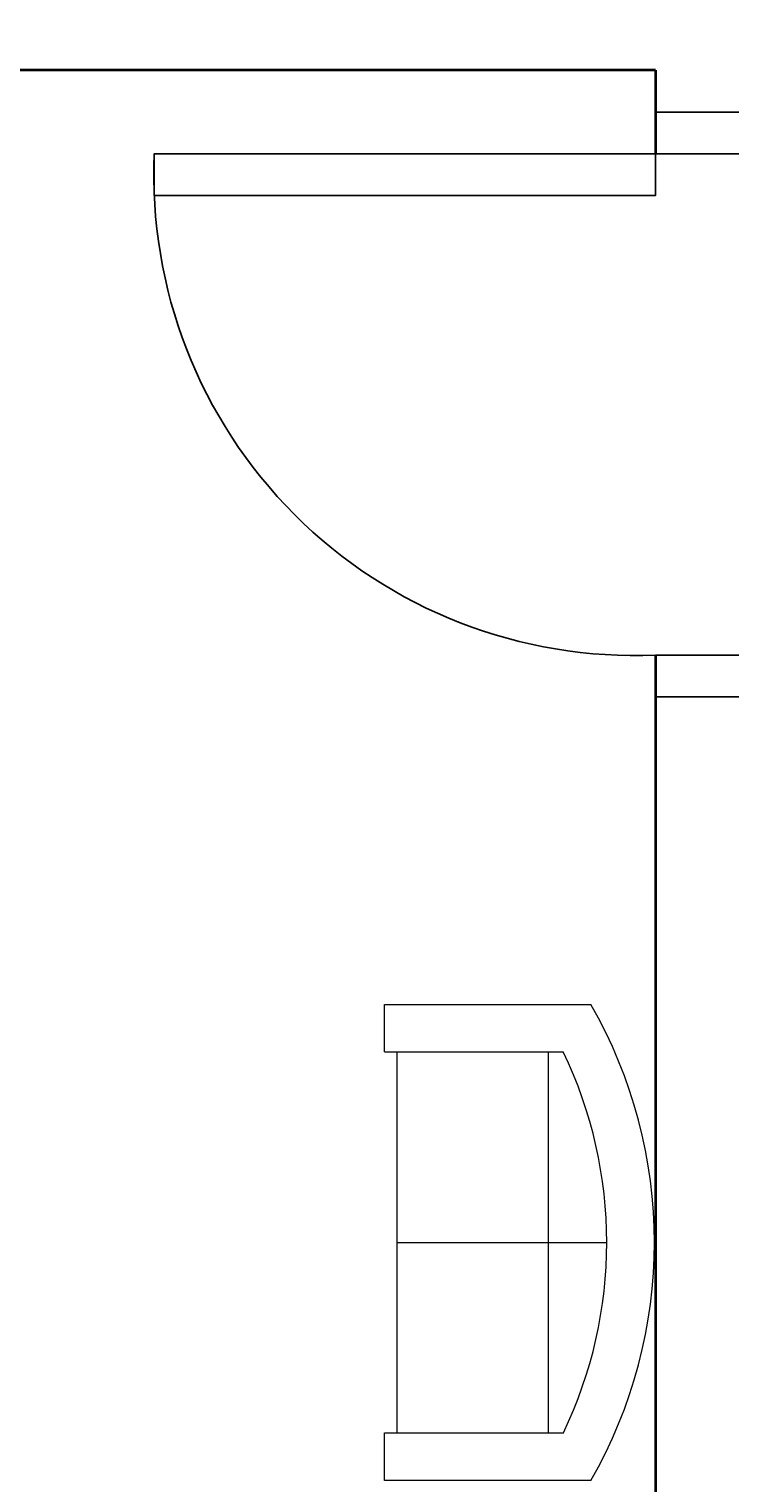
# Model space of a CAD drawing. Units: inches. Extents: x 4159 to 4826, y 299 to 1026.
# Tile 26 of 37: x 4402 to 4453, y 559 to 663. Entities that reach past the tile are written whole.
import ezdxf

# ---------------------------------------------------------------- set-up
doc = ezdxf.new("R2010")
doc.units = ezdxf.units.IN
for name, color, linetype, lineweight in [('A-ANNO-DIMS', 2, 'Continuous', 18), ('A-DOOR', 4, 'Continuous', 25), ('A-FURN', 8, 'Continuous', 18), ('A-WALL', 7, 'Continuous', 35)]:
    doc.layers.add(name, color=color, linetype=linetype, lineweight=lineweight)
doc.styles.get("Standard").update_dxf_attribs({"font": 'arial.ttf'})
doc.dimstyles.get("Standard").update_dxf_attribs({"dimtxt": 0.18, "dimasz": 0.18, "dimexe": 0.18, "dimexo": 0.0625, "dimgap": 0.09, "dimtad": 0, "dimtih": 1, "dimtoh": 1, "dimdec": 4, "dimzin": 0, "dimdsep": 46, "dimtxsty": 'Standard', "dimcen": 0.09, "dimadec": 0, "dimazin": 0, "dimtfac": 1, "dimtdec": 4, "dimtofl": 0, "dimtmove": 0, "dimatfit": 3, "dimfxl": 1, "dimtolj": 1, "dimtzin": 0, "dimarcsym": 0})

# ---------------------------------------------------------------- blocks, each defined once
blk = doc.blocks.new('Sofa - Roundback Loveseat 5 ft.')
for p, q in [((0, -32.44198), (0, -5.99998)), ((-24, -33.99998), (-24, -11.46958)), ((24.00004, -33.99998), (24.00004, -11.46958)), ((-23.9998, -13.38178), (23.99986, -13.38178)), ((-24, -32.44198), (24.00004, -32.44198))]:
    blk.add_line(p, q)
for points in [[(-24, -33.99998), (-30, -33.99998), (-30, -7.99998)], [(30.00004, -7.99998), (30.00004, -33.99998), (24.00004, -33.99998)]]:
    blk.add_lwpolyline(points)
for centre, radius, start, end in [((0, -60.24998), 60.24998, 60.13715, 119.8628), ((0, -61.38438), 55.38444, 64.32083, 115.6792)]:
    blk.add_arc(centre, radius, start, end)
blk = doc.blocks.new('DOOR-SWING-36IN')
blk.add_lwpolyline([(0, 0), (-3, 0), (-3, 36), (0, 36)], close=True)
blk.add_arc((-1.5, 1.5), 34.53, 87.5104, 182.4896)
blk = doc.blocks.new('DOOR-FRAME-36IN')
for p, q in [((0, 6), (0, 0)), ((3, 6), (3, 0)), ((39, 6), (39, 0)), ((42, 6), (42, 0))]:
    blk.add_line(p, q)
blk = doc.blocks.new('*D44')
at = {"layer": 'A-ANNO-DIMS', "color": 0, "lineweight": -2, "transparency": 16777216}
for p, q in [((4287.26, 963.09), (4158.88, 963.09)), ((4159.06, 962.91), (4159.06, 647.83)), ((4159.06, 332.38), (4159.06, 647.46)), ((4447.25, 332.2), (4158.88, 332.2))]:
    blk.add_line(p, q, dxfattribs=at)
at = {"layer": 'A-ANNO-DIMS', "color": 0, "transparency": 16777216}
for points in [[(4159.03, 962.91), (4159.09, 962.91), (4159.06, 963.09)], [(4159.03, 332.38), (4159.09, 332.38), (4159.06, 332.2)]]:
    blk.add_solid(points, dxfattribs=at)
at = {"layer": 'Defpoints', "color": 0, "transparency": 16777216}
for p in [(4287.33, 963.09), (4159.06, 332.2), (4447.31, 332.2)]:
    blk.add_point(p, dxfattribs=at)
at = {"layer": 'A-ANNO-DIMS', "color": 0, "transparency": 16777216, "insert": (4159.06, 647.64), "char_height": 0.18, "attachment_point": 5}
blk.add_mtext('\\A1;630.9', dxfattribs=at)

msp = doc.modelspace()

# ---------------------------------------------------------------- linework, layer by layer
at = {"layer": 'A-WALL'}
for p, q in [((4447.31, 660.254), (4201.31, 660.254)), ((4447.31, 660.254), (4447.31, 654.254)), ((4447.31, 618.254), (4447.31, 539.254))]:
    msp.add_line(p, q, dxfattribs=at)

# ---------------------------------------------------------------- block references
at = {"layer": 'A-DOOR'}
for name, p, rotation in [('DOOR-FRAME-36IN', (4453.31, 615.254), 90.0000000000003), ('DOOR-SWING-36IN', (4447.31, 654.254), 89.99999999999957)]:
    msp.add_blockref(name, p, dxfattribs=dict(at, rotation=rotation))
at = {"layer": 'A-FURN', "xscale": 0.5700533147329089, "yscale": 0.5700533147329089, "zscale": 0.5700533147329089, "rotation": 270}
msp.add_blockref('Sofa - Roundback Loveseat 5 ft.', (4447.235, 576.069), dxfattribs=at)

# ---------------------------------------------------------------- dimensions: what is measured, and where the dimension line sits
at = {"layer": 'A-ANNO-DIMS'}
dim = msp.add_linear_dim(base=(4159.06, 332.195), p1=(4287.326, 963.093), p2=(4447.31, 332.195), angle=90, dimstyle='Standard', override={"dimdec": 1, "dimlfac": 1, "dimrnd": 0, "dimzin": 0, "dimdsep": 46, "dimlunit": 2}, dxfattribs=at)
dim.commit()
dim.dimension.update_dxf_attribs({"geometry": '*D44', "text_midpoint": (4159.06, 647.644)})

doc.saveas('drawing.dxf')
